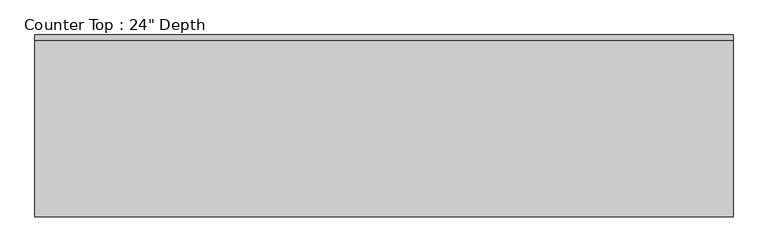
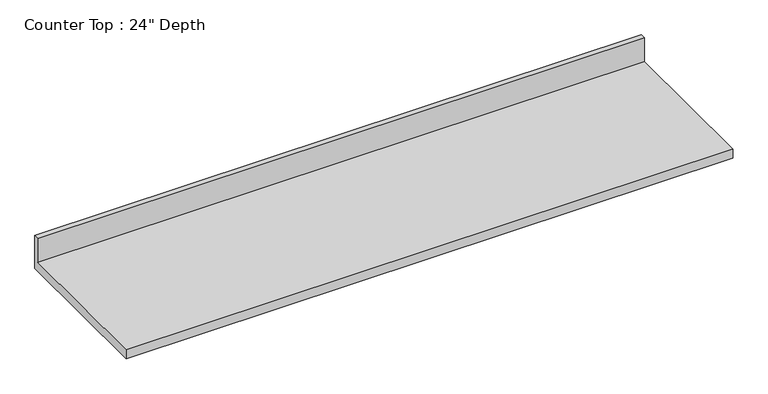
"""IFC4 building model written with IfcOpenShell, lengths in millimetres: furniture geometry."""

from ifc_helpers import new_model, si_unit, frame, origin, place, context, project, spatial, polyline, outline, extrude, source, transform, mapped, element, save


def furniture_deb1c5d1(model_context):
    return source(origin(), model_context, "Body", "SweptSolid", [
        extrude(outline(polyline([(0.0, 1016.0), (0.0, 876.3), (-635.0, 876.3), (-635.0, 914.4), (-19.05, 914.4), (-19.05, 1016.0), (0.0, 1016.0)])), frame((-1200.4622951, 0.0, 0.0), z_axis=(1.0, 0.0, 0.0), x_axis=(0.0, 1.0, 0.0)), (0.0, 0.0, 1.0), 2438.4),
    ])


if __name__ == "__main__":
    model = new_model("IFC4")
    model_context = context("Model", 3, world=origin())
    ifc_project = project(units=[si_unit("LENGTHUNIT", "METRE", prefix="MILLI")], contexts=[model_context])
    site = spatial("IfcSite", under=ifc_project)
    building = spatial("IfcBuilding", under=site)
    placement = place(None, origin())
    furniture_shape = furniture_deb1c5d1(model_context)
    element("IfcFurniture", 1, ObjectType="Counter Top : 24\" Depth", at=placement, inside=building, context=model_context, shape_type="MappedRepresentation", body=[
        mapped(furniture_shape, transform((0.0, 0.0, 0.0), x_axis=(1.0, 0.0, 0.0), y_axis=(0.0, 1.0, 0.0), z_axis=(0.0, 0.0, 1.0))),
    ])
    save(model, "model.ifc")

# Revit data of these elements
# Type "Counter Top : 24\" Depth"
#   Assembly Code = "C1030400"
#   Counter Thickness = 0' - 1 1/2"
#   Depth = 2' - 1"
#   Height = 3' - 0"
#   Length [instance default] = 8' - 0"
#   Counter Top Material = none
#   Default Elevation = 0
# Element 1 (IfcFurniture, "Counter Top : 24\" Depth")
#   Materials on its faces: "Counter Top"
# Materials
#   "Counter Top": class "Wood", colour RGB 226 177 128, transparency 0
